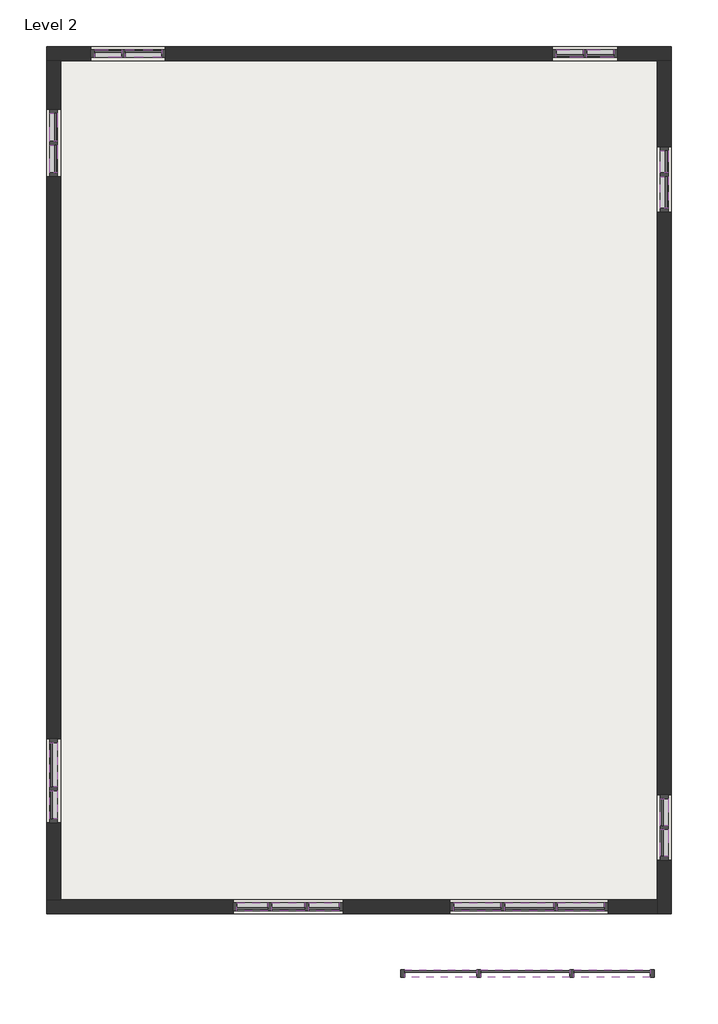
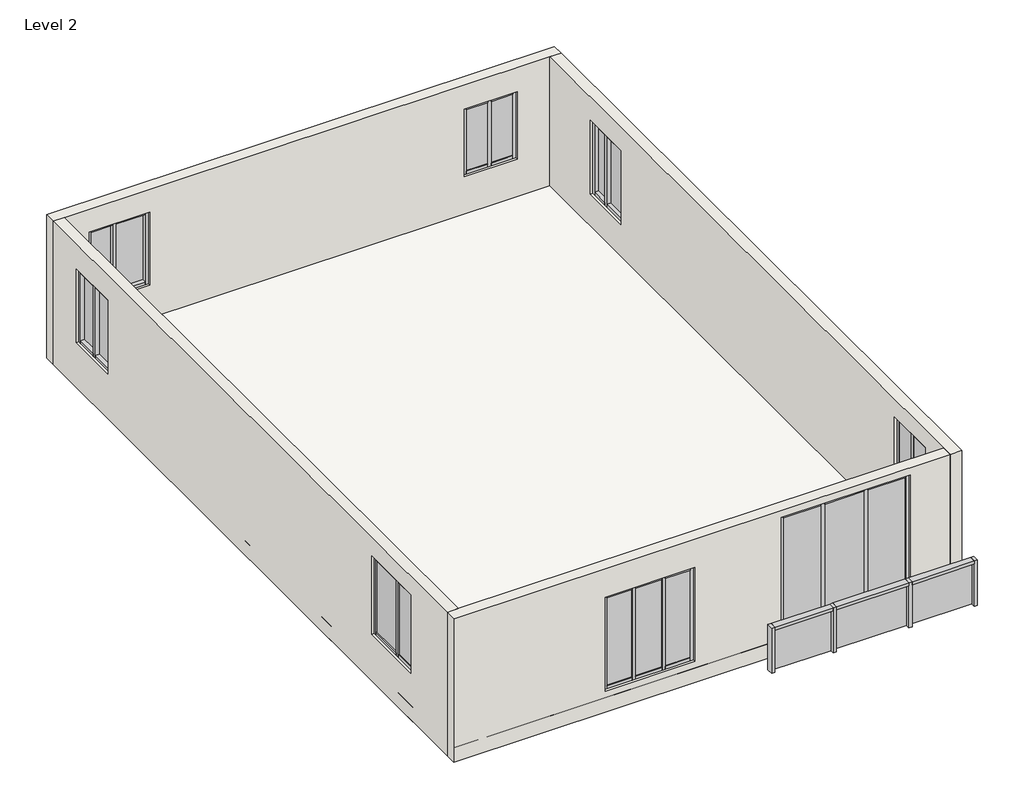
# One storey: 69 members, 21 plates, 4 walls, 1 roof.
"""IFC4 building model written with IfcOpenShell, lengths in millimetres."""

from ifc_helpers import new_model, si_unit, frame, origin, place, context, project, spatial, polyline, outline, extrude, faceted_brep, transform, mapped, element, save
from components import member_e5d39754, member_07406574, member_3ed29256, member_6fb4a552, member_97f07227, member_3e567bd2, member_843225dc, member_0b7646a3, member_1e2e73c0, member_6b6fe981, member_b1e1b578, member_5b6a755a, member_0486e582, member_4eea421a, member_9dbbeca1, member_3cfa9974, member_e7b97c4b, member_5535eeb3, member_7007ad49, member_cfa26838, member_5cb4264a, member_46f5bc36, member_d4df521d, member_0537779b, member_d36207d9, member_2d710983, member_80b18894, member_dd4241ee, member_fb497cbf, member_58cc8d1f, member_066849cb, member_d635bea1, system_panel_glazed_78e3b77e, system_panel_glazed_8adce2ad, system_panel_glazed_79a5eb44, system_panel_glazed_1572ce70, system_panel_glazed_a38fa740, system_panel_glazed_c088aa0a, system_panel_glazed_e446b74d, system_panel_glazed_482dc4ba, system_panel_glazed_bd259d29, system_panel_glazed_c39fb08b, system_panel_glazed_eabd6c1f, system_panel_glazed_831ab98e, system_panel_glazed_4b6d2a40, system_panel_glazed_d871acfc, system_panel_glazed_8bce9487, system_panel_glazed_361cf07d

model = new_model("IFC4")

# Units and contexts
model_context = context("Model", 3, world=origin())
ifc_project = project(units=[si_unit("LENGTHUNIT", "METRE", prefix="MILLI")], contexts=[model_context])

# Site, building, storey
site = spatial("IfcSite", under=ifc_project)
building = spatial("IfcBuilding", under=site)
storey = spatial("IfcBuildingStorey", under=building, Name="Level 2", Elevation=3048.0)

# Members
placement = place(None, origin())
member_shape = member_e5d39754(model_context)
element("IfcMember", 1, ObjectType="Rectangular Mullion : 2.5\" x 5\" rectangular", at=placement, inside=storey, context=model_context, shape_type="MappedRepresentation", body=[
    mapped(member_shape, transform((-15758.7624893, 1071.6959625, 5609.8739989), x_axis=(0.0, 0.0, 1.0), y_axis=(0.0, -1.0, 0.0), z_axis=(1.0, 0.0, 0.0))),
])
element("IfcMember", 2, ObjectType="Rectangular Mullion : 2.5\" x 5\" rectangular", at=placement, inside=storey, context=model_context, shape_type="MappedRepresentation", body=[
    mapped(member_shape, transform((-16349.3124893, 1071.6959625, 4052.5030277), x_axis=(0.0, 0.0, -1.0), y_axis=(0.0, -1.0, 0.0), z_axis=(-1.0, 0.0, 0.0))),
])
member_2_shape = member_07406574(model_context)
element("IfcMember", 3, ObjectType="Rectangular Mullion : 2.5\" x 5\" rectangular", at=placement, inside=storey, context=model_context, shape_type="MappedRepresentation", body=[
    mapped(member_2_shape, transform((-13356.3458226, -12872.9040375, 5485.7911654), x_axis=(0.0, 0.0, 1.0), y_axis=(0.0, 1.0, 0.0), z_axis=(-1.0, 0.0, 0.0))),
])
element("IfcMember", 4, ObjectType="Rectangular Mullion : 2.5\" x 5\" rectangular", at=placement, inside=storey, context=model_context, shape_type="MappedRepresentation", body=[
    mapped(member_2_shape, transform((-14526.8624893, -12872.9040375, 5485.7911654), x_axis=(0.0, 0.0, 1.0), y_axis=(0.0, 1.0, 0.0), z_axis=(-1.0, 0.0, 0.0))),
])
member_3_shape = member_3ed29256(model_context)
element("IfcMember", 5, ObjectType="Rectangular Mullion : 2.5\" x 5\" rectangular", at=placement, inside=storey, context=model_context, shape_type="MappedRepresentation", body=[
    mapped(member_3_shape, transform((-13957.479156, -12872.9040375, 5485.7911654), x_axis=(0.0, 0.0, 1.0), y_axis=(0.0, 1.0, 0.0), z_axis=(-1.0, 0.0, 0.0))),
])
element("IfcMember", 6, ObjectType="Rectangular Mullion : 2.5\" x 5\" rectangular", at=placement, inside=storey, context=model_context, shape_type="MappedRepresentation", body=[
    mapped(member_3_shape, transform((-13419.8458226, -12872.9040375, 3489.9238444), x_axis=(0.0, 0.0, -1.0), y_axis=(0.0, 1.0, 0.0), z_axis=(1.0, 0.0, 0.0))),
])
element("IfcMember", 7, ObjectType="Rectangular Mullion : 2.5\" x 5\" rectangular", at=placement, inside=storey, context=model_context, shape_type="MappedRepresentation", body=[
    mapped(member_2_shape, transform((-14020.979156, -12872.9040375, 3489.9238444), x_axis=(0.0, 0.0, -1.0), y_axis=(0.0, 1.0, 0.0), z_axis=(1.0, 0.0, 0.0))),
])
element("IfcMember", 8, ObjectType="Rectangular Mullion : 2.5\" x 5\" rectangular", at=placement, inside=storey, context=model_context, shape_type="MappedRepresentation", body=[
    mapped(member_2_shape, transform((-12850.4624893, -12872.9040375, 3489.9238444), x_axis=(0.0, 0.0, -1.0), y_axis=(0.0, 1.0, 0.0), z_axis=(1.0, 0.0, 0.0))),
])
member_4_shape = member_6fb4a552(model_context)
element("IfcMember", 9, ObjectType="Rectangular Mullion : 2.5\" x 5\" rectangular", at=placement, inside=storey, context=model_context, shape_type="MappedRepresentation", body=[
    mapped(member_4_shape, transform((-7541.8624893, -11609.2540375, 5711.9340524), x_axis=(0.0, 0.0, 1.0), y_axis=(1.0, 0.0, 0.0), z_axis=(0.0, 1.0, 0.0))),
])
element("IfcMember", 10, ObjectType="Rectangular Mullion : 2.5\" x 5\" rectangular", at=placement, inside=storey, context=model_context, shape_type="MappedRepresentation", body=[
    mapped(member_4_shape, transform((-7541.8624893, -11107.6040375, 5711.9340524), x_axis=(0.0, 0.0, 1.0), y_axis=(1.0, 0.0, 0.0), z_axis=(0.0, 1.0, 0.0))),
])
element("IfcMember", 11, ObjectType="Rectangular Mullion : 2.5\" x 5\" rectangular", at=placement, inside=storey, context=model_context, shape_type="MappedRepresentation", body=[
    mapped(member_4_shape, transform((-8805.5124893, 1071.6959625, 5579.9993984), x_axis=(0.0, 0.0, 1.0), y_axis=(0.0, 1.0, 0.0), z_axis=(-1.0, 0.0, 0.0))),
])
element("IfcMember", 12, ObjectType="Rectangular Mullion : 2.5\" x 5\" rectangular", at=placement, inside=storey, context=model_context, shape_type="MappedRepresentation", body=[
    mapped(member_4_shape, transform((-9307.1624893, 1071.6959625, 5579.9993984), x_axis=(0.0, 0.0, 1.0), y_axis=(0.0, 1.0, 0.0), z_axis=(-1.0, 0.0, 0.0))),
])
element("IfcMember", 13, ObjectType="Rectangular Mullion : 2.5\" x 5\" rectangular", at=placement, inside=storey, context=model_context, shape_type="MappedRepresentation", body=[
    mapped(member_4_shape, transform((-16412.8124893, 1071.6959625, 5609.8739989), x_axis=(0.0, 0.0, 1.0), y_axis=(0.0, -1.0, 0.0), z_axis=(1.0, 0.0, 0.0))),
])
member_5_shape = member_97f07227(model_context)
element("IfcMember", 14, ObjectType="Rectangular Mullion : 2.5\" x 5\" rectangular", at=placement, inside=storey, context=model_context, shape_type="MappedRepresentation", body=[
    mapped(member_5_shape, transform((-7541.8624893, -11577.5040375, 4161.6494696), x_axis=(0.0, 1.0, 0.0), y_axis=(1.0, 0.0, 0.0), z_axis=(0.0, 0.0, -1.0))),
])
element("IfcMember", 15, ObjectType="Rectangular Mullion : 2.5\" x 5\" rectangular", at=placement, inside=storey, context=model_context, shape_type="MappedRepresentation", body=[
    mapped(member_4_shape, transform((-7541.8624893, -11545.7540375, 4161.6494696), x_axis=(0.0, 0.0, -1.0), y_axis=(1.0, 0.0, 0.0), z_axis=(0.0, -1.0, 0.0))),
])
element("IfcMember", 16, ObjectType="Rectangular Mullion : 2.5\" x 5\" rectangular", at=placement, inside=storey, context=model_context, shape_type="MappedRepresentation", body=[
    mapped(member_4_shape, transform((-7541.8624893, -12047.4040375, 4161.6494696), x_axis=(0.0, 0.0, -1.0), y_axis=(1.0, 0.0, 0.0), z_axis=(0.0, -1.0, 0.0))),
])
element("IfcMember", 17, ObjectType="Rectangular Mullion : 2.5\" x 5\" rectangular", at=placement, inside=storey, context=model_context, shape_type="MappedRepresentation", body=[
    mapped(member_4_shape, transform((-8869.0124893, 1071.6959625, 4146.229298), x_axis=(0.0, 0.0, -1.0), y_axis=(0.0, 1.0, 0.0), z_axis=(1.0, 0.0, 0.0))),
])
element("IfcMember", 18, ObjectType="Rectangular Mullion : 2.5\" x 5\" rectangular", at=placement, inside=storey, context=model_context, shape_type="MappedRepresentation", body=[
    mapped(member_4_shape, transform((-8367.3624893, 1071.6959625, 4146.229298), x_axis=(0.0, 0.0, -1.0), y_axis=(0.0, 1.0, 0.0), z_axis=(1.0, 0.0, 0.0))),
])
element("IfcMember", 19, ObjectType="Rectangular Mullion : 2.5\" x 5\" rectangular", at=placement, inside=storey, context=model_context, shape_type="MappedRepresentation", body=[
    mapped(member_4_shape, transform((-16850.9624893, 1071.6959625, 4052.5030277), x_axis=(0.0, 0.0, -1.0), y_axis=(0.0, -1.0, 0.0), z_axis=(-1.0, 0.0, 0.0))),
])
member_6_shape = member_3e567bd2(model_context)
element("IfcMember", 20, ObjectType="Rectangular Mullion : 2.5\" x 5\" rectangular", at=placement, inside=storey, context=model_context, shape_type="MappedRepresentation", body=[
    mapped(member_6_shape, transform((-7541.8624893, -11044.1040375, 4161.6494696), x_axis=(0.0, 1.0, 0.0), y_axis=(1.0, 0.0, 0.0), z_axis=(0.0, 0.0, -1.0))),
])
element("IfcMember", 21, ObjectType="Rectangular Mullion : 2.5\" x 5\" rectangular", at=placement, inside=storey, context=model_context, shape_type="MappedRepresentation", body=[
    mapped(member_6_shape, transform((-7541.8624893, -12110.9040375, 5711.9340524), x_axis=(0.0, -1.0, 0.0), y_axis=(1.0, 0.0, 0.0), z_axis=(0.0, 0.0, 1.0))),
])
member_7_shape = member_843225dc(model_context)
element("IfcMember", 22, ObjectType="Rectangular Mullion : 2.5\" x 5\" rectangular", at=placement, inside=storey, context=model_context, shape_type="MappedRepresentation", body=[
    mapped(member_7_shape, transform((-7541.8624893, -877.7540375, 5599.6032414), x_axis=(0.0, 0.0, 1.0), y_axis=(-1.0, 0.0, 0.0), z_axis=(0.0, -1.0, 0.0))),
])
member_8_shape = member_0b7646a3(model_context)
element("IfcMember", 23, ObjectType="Rectangular Mullion : 2.5\" x 5\" rectangular", at=placement, inside=storey, context=model_context, shape_type="MappedRepresentation", body=[
    mapped(member_8_shape, transform((-7541.8624893, -1455.6040375, 5599.6032414), x_axis=(0.0, 0.0, 1.0), y_axis=(-1.0, 0.0, 0.0), z_axis=(0.0, -1.0, 0.0))),
])
member_9_shape = member_1e2e73c0(model_context)
element("IfcMember", 24, ObjectType="Rectangular Mullion : 2.5\" x 5\" rectangular", at=placement, inside=storey, context=model_context, shape_type="MappedRepresentation", body=[
    mapped(member_9_shape, transform((-7541.8624893, -909.5040375, 4029.8396627), x_axis=(0.0, -1.0, 0.0), y_axis=(-1.0, 0.0, 0.0), z_axis=(0.0, 0.0, -1.0))),
])
element("IfcMember", 25, ObjectType="Rectangular Mullion : 2.5\" x 5\" rectangular", at=placement, inside=storey, context=model_context, shape_type="MappedRepresentation", body=[
    mapped(member_8_shape, transform((-7541.8624893, -941.2540375, 4029.8396627), x_axis=(0.0, 0.0, -1.0), y_axis=(-1.0, 0.0, 0.0), z_axis=(0.0, 1.0, 0.0))),
])
element("IfcMember", 26, ObjectType="Rectangular Mullion : 2.5\" x 5\" rectangular", at=placement, inside=storey, context=model_context, shape_type="MappedRepresentation", body=[
    mapped(member_7_shape, transform((-7541.8624893, -515.8040375, 4029.8396627), x_axis=(0.0, 0.0, -1.0), y_axis=(-1.0, 0.0, 0.0), z_axis=(0.0, 1.0, 0.0))),
])
member_10_shape = member_6b6fe981(model_context)
element("IfcMember", 27, ObjectType="Rectangular Mullion : 2.5\" x 5\" rectangular", at=placement, inside=storey, context=model_context, shape_type="MappedRepresentation", body=[
    mapped(member_10_shape, transform((-7541.8624893, -452.3040375, 5599.6032414), x_axis=(0.0, 1.0, 0.0), y_axis=(-1.0, 0.0, 0.0), z_axis=(0.0, 0.0, 1.0))),
])
element("IfcMember", 28, ObjectType="Rectangular Mullion : 2.5\" x 5\" rectangular", at=placement, inside=storey, context=model_context, shape_type="MappedRepresentation", body=[
    mapped(member_10_shape, transform((-7541.8624893, -1519.1040375, 4029.8396627), x_axis=(0.0, -1.0, 0.0), y_axis=(-1.0, 0.0, 0.0), z_axis=(0.0, 0.0, -1.0))),
])
member_11_shape = member_b1e1b578(model_context)
element("IfcMember", 29, ObjectType="Rectangular Mullion : 2.5\" x 5\" rectangular", at=placement, inside=storey, context=model_context, shape_type="MappedRepresentation", body=[
    mapped(member_11_shape, transform((-8837.2624893, 1071.6959625, 4146.229298), x_axis=(-1.0, 0.0, 0.0), y_axis=(0.0, 1.0, 0.0), z_axis=(0.0, 0.0, -1.0))),
])
member_12_shape = member_5b6a755a(model_context)
element("IfcMember", 30, ObjectType="Rectangular Mullion : 2.5\" x 5\" rectangular", at=placement, inside=storey, context=model_context, shape_type="MappedRepresentation", body=[
    mapped(member_12_shape, transform((-9370.6624893, 1071.6959625, 4146.229298), x_axis=(-1.0, 0.0, 0.0), y_axis=(0.0, 1.0, 0.0), z_axis=(0.0, 0.0, -1.0))),
])
element("IfcMember", 31, ObjectType="Rectangular Mullion : 2.5\" x 5\" rectangular", at=placement, inside=storey, context=model_context, shape_type="MappedRepresentation", body=[
    mapped(member_12_shape, transform((-8303.8624893, 1071.6959625, 5579.9993984), x_axis=(1.0, 0.0, 0.0), y_axis=(0.0, 1.0, 0.0), z_axis=(0.0, 0.0, 1.0))),
])
member_13_shape = member_0486e582(model_context)
element("IfcMember", 32, ObjectType="Rectangular Mullion : 2.5\" x 5\" rectangular", at=placement, inside=storey, context=model_context, shape_type="MappedRepresentation", body=[
    mapped(member_13_shape, transform((-16381.0624893, 1071.6959625, 4052.5030277), x_axis=(1.0, 0.0, 0.0), y_axis=(0.0, -1.0, 0.0), z_axis=(0.0, 0.0, -1.0))),
])
member_14_shape = member_4eea421a(model_context)
element("IfcMember", 33, ObjectType="Rectangular Mullion : 2.5\" x 5\" rectangular", at=placement, inside=storey, context=model_context, shape_type="MappedRepresentation", body=[
    mapped(member_14_shape, transform((-16914.4624893, 1071.6959625, 5609.8739989), x_axis=(-1.0, 0.0, 0.0), y_axis=(0.0, -1.0, 0.0), z_axis=(0.0, 0.0, 1.0))),
])
element("IfcMember", 34, ObjectType="Rectangular Mullion : 2.5\" x 5\" rectangular", at=placement, inside=storey, context=model_context, shape_type="MappedRepresentation", body=[
    mapped(member_14_shape, transform((-15695.2624893, 1071.6959625, 4052.5030277), x_axis=(1.0, 0.0, 0.0), y_axis=(0.0, -1.0, 0.0), z_axis=(0.0, 0.0, -1.0))),
])
member_15_shape = member_9dbbeca1(model_context)
element("IfcMember", 35, ObjectType="Rectangular Mullion : 2.5\" x 5\" rectangular", at=placement, inside=storey, context=model_context, shape_type="MappedRepresentation", body=[
    mapped(member_15_shape, transform((-17524.0624893, -360.2290375, 5564.8264528), x_axis=(0.0, 0.0, 1.0), y_axis=(-1.0, 0.0, 0.0), z_axis=(0.0, -1.0, 0.0))),
])
element("IfcMember", 36, ObjectType="Rectangular Mullion : 2.5\" x 5\" rectangular", at=placement, inside=storey, context=model_context, shape_type="MappedRepresentation", body=[
    mapped(member_15_shape, transform((-17524.0624893, -877.7540375, 5564.8264528), x_axis=(0.0, 0.0, 1.0), y_axis=(-1.0, 0.0, 0.0), z_axis=(0.0, -1.0, 0.0))),
])
member_16_shape = member_3cfa9974(model_context)
element("IfcMember", 37, ObjectType="Rectangular Mullion : 2.5\" x 5\" rectangular", at=placement, inside=storey, context=model_context, shape_type="MappedRepresentation", body=[
    mapped(member_16_shape, transform((-17524.0624893, -391.9790375, 3995.7999113), x_axis=(0.0, -1.0, 0.0), y_axis=(-1.0, 0.0, 0.0), z_axis=(0.0, 0.0, -1.0))),
])
element("IfcMember", 38, ObjectType="Rectangular Mullion : 2.5\" x 5\" rectangular", at=placement, inside=storey, context=model_context, shape_type="MappedRepresentation", body=[
    mapped(member_15_shape, transform((-17524.0624893, -423.7290375, 3995.7999113), x_axis=(0.0, 0.0, -1.0), y_axis=(-1.0, 0.0, 0.0), z_axis=(0.0, 1.0, 0.0))),
])
element("IfcMember", 39, ObjectType="Rectangular Mullion : 2.5\" x 5\" rectangular", at=placement, inside=storey, context=model_context, shape_type="MappedRepresentation", body=[
    mapped(member_15_shape, transform((-17524.0624893, 93.7959625, 3995.7999113), x_axis=(0.0, 0.0, -1.0), y_axis=(-1.0, 0.0, 0.0), z_axis=(0.0, 1.0, 0.0))),
])
member_17_shape = member_e7b97c4b(model_context)
element("IfcMember", 40, ObjectType="Rectangular Mullion : 2.5\" x 5\" rectangular", at=placement, inside=storey, context=model_context, shape_type="MappedRepresentation", body=[
    mapped(member_17_shape, transform((-17524.0624893, -941.2540375, 3995.7999113), x_axis=(0.0, -1.0, 0.0), y_axis=(-1.0, 0.0, 0.0), z_axis=(0.0, 0.0, -1.0))),
])
element("IfcMember", 41, ObjectType="Rectangular Mullion : 2.5\" x 5\" rectangular", at=placement, inside=storey, context=model_context, shape_type="MappedRepresentation", body=[
    mapped(member_17_shape, transform((-17524.0624893, 157.2959625, 5564.8264528), x_axis=(0.0, 1.0, 0.0), y_axis=(-1.0, 0.0, 0.0), z_axis=(0.0, 0.0, 1.0))),
])
member_18_shape = member_5535eeb3(model_context)
element("IfcMember", 42, ObjectType="Rectangular Mullion : 2.5\" x 5\" rectangular", at=placement, inside=storey, context=model_context, shape_type="MappedRepresentation", body=[
    mapped(member_18_shape, transform((-17524.0624893, -10974.2540375, 5698.7553745), x_axis=(0.0, 0.0, 1.0), y_axis=(1.0, 0.0, 0.0), z_axis=(0.0, 1.0, 0.0))),
])
member_19_shape = member_7007ad49(model_context)
element("IfcMember", 43, ObjectType="Rectangular Mullion : 2.5\" x 5\" rectangular", at=placement, inside=storey, context=model_context, shape_type="MappedRepresentation", body=[
    mapped(member_19_shape, transform((-17524.0624893, -10193.2040375, 5698.7553745), x_axis=(0.0, 0.0, 1.0), y_axis=(1.0, 0.0, 0.0), z_axis=(0.0, 1.0, 0.0))),
])
member_20_shape = member_cfa26838(model_context)
element("IfcMember", 44, ObjectType="Rectangular Mullion : 2.5\" x 5\" rectangular", at=placement, inside=storey, context=model_context, shape_type="MappedRepresentation", body=[
    mapped(member_20_shape, transform((-17524.0624893, -10942.5040375, 4032.9560025), x_axis=(0.0, 1.0, 0.0), y_axis=(1.0, 0.0, 0.0), z_axis=(0.0, 0.0, -1.0))),
])
element("IfcMember", 45, ObjectType="Rectangular Mullion : 2.5\" x 5\" rectangular", at=placement, inside=storey, context=model_context, shape_type="MappedRepresentation", body=[
    mapped(member_19_shape, transform((-17524.0624893, -10910.7540375, 4032.9560025), x_axis=(0.0, 0.0, -1.0), y_axis=(1.0, 0.0, 0.0), z_axis=(0.0, -1.0, 0.0))),
])
element("IfcMember", 46, ObjectType="Rectangular Mullion : 2.5\" x 5\" rectangular", at=placement, inside=storey, context=model_context, shape_type="MappedRepresentation", body=[
    mapped(member_18_shape, transform((-17524.0624893, -11437.8040375, 4032.9560025), x_axis=(0.0, 0.0, -1.0), y_axis=(1.0, 0.0, 0.0), z_axis=(0.0, -1.0, 0.0))),
])
member_21_shape = member_5cb4264a(model_context)
element("IfcMember", 47, ObjectType="Rectangular Mullion : 2.5\" x 5\" rectangular", at=placement, inside=storey, context=model_context, shape_type="MappedRepresentation", body=[
    mapped(member_21_shape, transform((-17524.0624893, -11501.3040375, 5698.7553745), x_axis=(0.0, -1.0, 0.0), y_axis=(1.0, 0.0, 0.0), z_axis=(0.0, 0.0, 1.0))),
])
element("IfcMember", 48, ObjectType="Rectangular Mullion : 2.5\" x 5\" rectangular", at=placement, inside=storey, context=model_context, shape_type="MappedRepresentation", body=[
    mapped(member_21_shape, transform((-17524.0624893, -10129.7040375, 4032.9560025), x_axis=(0.0, 1.0, 0.0), y_axis=(1.0, 0.0, 0.0), z_axis=(0.0, 0.0, -1.0))),
])
member_22_shape = member_46f5bc36(model_context)
element("IfcMember", 49, ObjectType="Rectangular Mullion : 2.5\" x 5\" rectangular", at=placement, inside=storey, context=model_context, shape_type="MappedRepresentation", body=[
    mapped(member_22_shape, transform((-9288.1124893, -12872.9040375, 5944.1398762), x_axis=(0.0, 0.0, 1.0), y_axis=(0.0, 1.0, 0.0), z_axis=(-1.0, 0.0, 0.0))),
])
element("IfcMember", 50, ObjectType="Rectangular Mullion : 2.5\" x 5\" rectangular", at=placement, inside=storey, context=model_context, shape_type="MappedRepresentation", body=[
    mapped(member_22_shape, transform((-10983.5624893, -12872.9040375, 5944.1398762), x_axis=(0.0, 0.0, 1.0), y_axis=(0.0, 1.0, 0.0), z_axis=(-1.0, 0.0, 0.0))),
])
member_23_shape = member_d4df521d(model_context)
element("IfcMember", 51, ObjectType="Rectangular Mullion : 2.5\" x 5\" rectangular", at=placement, inside=storey, context=model_context, shape_type="MappedRepresentation", body=[
    mapped(member_23_shape, transform((-10183.4624893, -12872.9040375, 3475.7949453), x_axis=(-1.0, 0.0, 0.0), y_axis=(0.0, 1.0, 0.0), z_axis=(0.0, 0.0, -1.0))),
])
element("IfcMember", 52, ObjectType="Rectangular Mullion : 2.5\" x 5\" rectangular", at=placement, inside=storey, context=model_context, shape_type="MappedRepresentation", body=[
    mapped(member_23_shape, transform((-9319.8624893, -12872.9040375, 3475.7949453), x_axis=(-1.0, 0.0, 0.0), y_axis=(0.0, 1.0, 0.0), z_axis=(0.0, 0.0, -1.0))),
])
element("IfcMember", 53, ObjectType="Rectangular Mullion : 2.5\" x 5\" rectangular", at=placement, inside=storey, context=model_context, shape_type="MappedRepresentation", body=[
    mapped(member_22_shape, transform((-10215.2124893, -12872.9040375, 3475.7949453), x_axis=(0.0, 0.0, -1.0), y_axis=(0.0, 1.0, 0.0), z_axis=(1.0, 0.0, 0.0))),
])
element("IfcMember", 54, ObjectType="Rectangular Mullion : 2.5\" x 5\" rectangular", at=placement, inside=storey, context=model_context, shape_type="MappedRepresentation", body=[
    mapped(member_22_shape, transform((-8519.7624893, -12872.9040375, 3475.7949453), x_axis=(0.0, 0.0, -1.0), y_axis=(0.0, 1.0, 0.0), z_axis=(1.0, 0.0, 0.0))),
])
member_24_shape = member_0537779b(model_context)
element("IfcMember", 55, ObjectType="Rectangular Mullion : 2.5\" x 5\" rectangular", at=placement, inside=storey, context=model_context, shape_type="MappedRepresentation", body=[
    mapped(member_24_shape, transform((-11047.0624893, -12872.9040375, 3475.7949453), x_axis=(-1.0, 0.0, 0.0), y_axis=(0.0, 1.0, 0.0), z_axis=(0.0, 0.0, -1.0))),
])
member_25_shape = member_d36207d9(model_context)
element("IfcMember", 56, ObjectType="Rectangular Mullion : 2.5\" x 5\" rectangular", at=placement, inside=storey, context=model_context, shape_type="MappedRepresentation", body=[
    mapped(member_25_shape, transform((-10151.7124893, -12872.9040375, 5944.1398762), x_axis=(0.0, 0.0, 1.0), y_axis=(0.0, 1.0, 0.0), z_axis=(-1.0, 0.0, 0.0))),
])
element("IfcMember", 57, ObjectType="Rectangular Mullion : 2.5\" x 5\" rectangular", at=placement, inside=storey, context=model_context, shape_type="MappedRepresentation", body=[
    mapped(member_25_shape, transform((-9351.6124893, -12872.9040375, 3475.7949453), x_axis=(0.0, 0.0, -1.0), y_axis=(0.0, 1.0, 0.0), z_axis=(1.0, 0.0, 0.0))),
])
element("IfcMember", 58, ObjectType="Rectangular Mullion : 2.5\" x 5\" rectangular", at=placement, inside=storey, context=model_context, shape_type="MappedRepresentation", body=[
    mapped(member_24_shape, transform((-8456.2624893, -12872.9040375, 5944.1398762), x_axis=(1.0, 0.0, 0.0), y_axis=(0.0, 1.0, 0.0), z_axis=(0.0, 0.0, 1.0))),
])
member_26_shape = member_2d710983(model_context)
element("IfcMember", 59, ObjectType="Rectangular Mullion : 2.5\" x 5\" rectangular", at=placement, inside=storey, context=model_context, shape_type="MappedRepresentation", body=[
    mapped(member_26_shape, transform((-13989.229156, -12872.9040375, 3489.9238444), x_axis=(-1.0, 0.0, 0.0), y_axis=(0.0, 1.0, 0.0), z_axis=(0.0, 0.0, -1.0))),
])
element("IfcMember", 60, ObjectType="Rectangular Mullion : 2.5\" x 5\" rectangular", at=placement, inside=storey, context=model_context, shape_type="MappedRepresentation", body=[
    mapped(member_26_shape, transform((-13388.0958226, -12872.9040375, 3489.9238444), x_axis=(-1.0, 0.0, 0.0), y_axis=(0.0, 1.0, 0.0), z_axis=(0.0, 0.0, -1.0))),
])
member_27_shape = member_80b18894(model_context)
element("IfcMember", 61, ObjectType="Rectangular Mullion : 2.5\" x 5\" rectangular", at=placement, inside=storey, context=model_context, shape_type="MappedRepresentation", body=[
    mapped(member_27_shape, transform((-12786.9624893, -12872.9040375, 5485.7911654), x_axis=(1.0, 0.0, 0.0), y_axis=(0.0, 1.0, 0.0), z_axis=(0.0, 0.0, 1.0))),
])
element("IfcMember", 62, ObjectType="Rectangular Mullion : 2.5\" x 5\" rectangular", at=placement, inside=storey, context=model_context, shape_type="MappedRepresentation", body=[
    mapped(member_27_shape, transform((-14590.3624893, -12872.9040375, 3489.9238444), x_axis=(-1.0, 0.0, 0.0), y_axis=(0.0, 1.0, 0.0), z_axis=(0.0, 0.0, -1.0))),
])
member_28_shape = member_dd4241ee(model_context)
element("IfcMember", 63, ObjectType="Rectangular Mullion : 2.5\" x 5\" rectangular", at=placement, inside=storey, context=model_context, shape_type="MappedRepresentation", body=[
    mapped(member_28_shape, transform((-11847.1624893, -13965.1040375, 4500.0986575), x_axis=(-1.0, 0.0, 0.0), y_axis=(0.0, -1.0, 0.0), z_axis=(0.0, 0.0, 1.0))),
])
member_29_shape = member_fb497cbf(model_context)
element("IfcMember", 64, ObjectType="Rectangular Mullion : 2.5\" x 5\" rectangular", at=placement, inside=storey, context=model_context, shape_type="MappedRepresentation", body=[
    mapped(member_29_shape, transform((-10608.9124893, -13965.1040375, 4500.0986575), x_axis=(0.0, 0.0, 1.0), y_axis=(0.0, -1.0, 0.0), z_axis=(1.0, 0.0, 0.0))),
])
member_30_shape = member_58cc8d1f(model_context)
element("IfcMember", 65, ObjectType="Rectangular Mullion : 2.5\" x 5\" rectangular", at=placement, inside=storey, context=model_context, shape_type="MappedRepresentation", body=[
    mapped(member_30_shape, transform((-10577.1624893, -13965.1040375, 3539.2949453), x_axis=(1.0, 0.0, 0.0), y_axis=(0.0, -1.0, 0.0), z_axis=(0.0, 0.0, -1.0))),
])
element("IfcMember", 66, ObjectType="Rectangular Mullion : 2.5\" x 5\" rectangular", at=placement, inside=storey, context=model_context, shape_type="MappedRepresentation", body=[
    mapped(member_30_shape, transform((-9055.2871232, -13965.1040375, 3539.2949453), x_axis=(1.0, 0.0, 0.0), y_axis=(0.0, -1.0, 0.0), z_axis=(0.0, 0.0, -1.0))),
])
member_31_shape = member_066849cb(model_context)
element("IfcMember", 67, ObjectType="Rectangular Mullion : 2.5\" x 5\" rectangular", at=placement, inside=storey, context=model_context, shape_type="MappedRepresentation", body=[
    mapped(member_31_shape, transform((-9087.0371232, -13965.1040375, 4500.0986575), x_axis=(0.0, 0.0, 1.0), y_axis=(0.0, -1.0, 0.0), z_axis=(1.0, 0.0, 0.0))),
])
member_32_shape = member_d635bea1(model_context)
element("IfcMember", 68, ObjectType="Rectangular Mullion : 2.5\" x 5\" rectangular", at=placement, inside=storey, context=model_context, shape_type="MappedRepresentation", body=[
    mapped(member_32_shape, transform((-7772.5871232, -13965.1040375, 4500.0986575), x_axis=(0.0, 0.0, 1.0), y_axis=(0.0, -1.0, 0.0), z_axis=(1.0, 0.0, 0.0))),
])
element("IfcMember", 69, ObjectType="Rectangular Mullion : 2.5\" x 5\" rectangular", at=placement, inside=storey, context=model_context, shape_type="MappedRepresentation", body=[
    mapped(member_28_shape, transform((-7709.0871232, -13965.1040375, 3539.2949453), x_axis=(1.0, 0.0, 0.0), y_axis=(0.0, -1.0, 0.0), z_axis=(0.0, 0.0, -1.0))),
])

# Plates
system_panel_glazed_shape = system_panel_glazed_78e3b77e(model_context)
element("IfcPlate", 70, ObjectType="System Panel : Glazed", at=placement, inside=storey, context=model_context, shape_type="MappedRepresentation", body=[
    mapped(system_panel_glazed_shape, transform((-7541.8624893, -11828.3290375, 4225.1494696), x_axis=(0.0, 1.0, 0.0), y_axis=(-1.0, 0.0, 0.0), z_axis=(0.0, 0.0, 1.0))),
])
element("IfcPlate", 71, ObjectType="System Panel : Glazed", at=placement, inside=storey, context=model_context, shape_type="MappedRepresentation", body=[
    mapped(system_panel_glazed_shape, transform((-7541.8624893, -11326.6790375, 4225.1494696), x_axis=(0.0, 1.0, 0.0), y_axis=(-1.0, 0.0, 0.0), z_axis=(0.0, 0.0, 1.0))),
])
system_panel_glazed_2_shape = system_panel_glazed_8adce2ad(model_context)
element("IfcPlate", 72, ObjectType="System Panel : Glazed", at=placement, inside=storey, context=model_context, shape_type="MappedRepresentation", body=[
    mapped(system_panel_glazed_2_shape, transform((-7541.8624893, -696.7790375, 4093.3396627), x_axis=(0.0, -1.0, 0.0), y_axis=(1.0, 0.0, 0.0), z_axis=(0.0, 0.0, 1.0))),
])
system_panel_glazed_3_shape = system_panel_glazed_79a5eb44(model_context)
element("IfcPlate", 73, ObjectType="System Panel : Glazed", at=placement, inside=storey, context=model_context, shape_type="MappedRepresentation", body=[
    mapped(system_panel_glazed_3_shape, transform((-7541.8624893, -1198.4290375, 4093.3396627), x_axis=(0.0, -1.0, 0.0), y_axis=(1.0, 0.0, 0.0), z_axis=(0.0, 0.0, 1.0))),
])
system_panel_glazed_4_shape = system_panel_glazed_1572ce70(model_context)
element("IfcPlate", 74, ObjectType="System Panel : Glazed", at=placement, inside=storey, context=model_context, shape_type="MappedRepresentation", body=[
    mapped(system_panel_glazed_4_shape, transform((-8586.4374893, 1071.6959625, 4209.729298), x_axis=(-1.0, 0.0, 0.0), y_axis=(0.0, -1.0, 0.0), z_axis=(0.0, 0.0, 1.0))),
])
element("IfcPlate", 75, ObjectType="System Panel : Glazed", at=placement, inside=storey, context=model_context, shape_type="MappedRepresentation", body=[
    mapped(system_panel_glazed_4_shape, transform((-9088.0874893, 1071.6959625, 4209.729298), x_axis=(-1.0, 0.0, 0.0), y_axis=(0.0, -1.0, 0.0), z_axis=(0.0, 0.0, 1.0))),
])
system_panel_glazed_5_shape = system_panel_glazed_a38fa740(model_context)
element("IfcPlate", 76, ObjectType="System Panel : Glazed", at=placement, inside=storey, context=model_context, shape_type="MappedRepresentation", body=[
    mapped(system_panel_glazed_5_shape, transform((-16631.8874893, 1071.6959625, 4116.0030277), x_axis=(1.0, 0.0, 0.0), y_axis=(0.0, 1.0, 0.0), z_axis=(0.0, 0.0, 1.0))),
])
system_panel_glazed_6_shape = system_panel_glazed_c088aa0a(model_context)
element("IfcPlate", 77, ObjectType="System Panel : Glazed", at=placement, inside=storey, context=model_context, shape_type="MappedRepresentation", body=[
    mapped(system_panel_glazed_6_shape, transform((-16054.0374893, 1071.6959625, 4116.0030277), x_axis=(1.0, 0.0, 0.0), y_axis=(0.0, 1.0, 0.0), z_axis=(0.0, 0.0, 1.0))),
])
system_panel_glazed_7_shape = system_panel_glazed_e446b74d(model_context)
element("IfcPlate", 78, ObjectType="System Panel : Glazed", at=placement, inside=storey, context=model_context, shape_type="MappedRepresentation", body=[
    mapped(system_panel_glazed_7_shape, transform((-17524.0624893, -133.2165375, 4059.2999113), x_axis=(0.0, -1.0, 0.0), y_axis=(1.0, 0.0, 0.0), z_axis=(0.0, 0.0, 1.0))),
])
element("IfcPlate", 79, ObjectType="System Panel : Glazed", at=placement, inside=storey, context=model_context, shape_type="MappedRepresentation", body=[
    mapped(system_panel_glazed_7_shape, transform((-17524.0624893, -650.7415375, 4059.2999113), x_axis=(0.0, -1.0, 0.0), y_axis=(1.0, 0.0, 0.0), z_axis=(0.0, 0.0, 1.0))),
])
system_panel_glazed_8_shape = system_panel_glazed_482dc4ba(model_context)
element("IfcPlate", 80, ObjectType="System Panel : Glazed", at=placement, inside=storey, context=model_context, shape_type="MappedRepresentation", body=[
    mapped(system_panel_glazed_8_shape, transform((-17524.0624893, -11206.0290375, 4096.4560025), x_axis=(0.0, 1.0, 0.0), y_axis=(-1.0, 0.0, 0.0), z_axis=(0.0, 0.0, 1.0))),
])
system_panel_glazed_9_shape = system_panel_glazed_bd259d29(model_context)
element("IfcPlate", 81, ObjectType="System Panel : Glazed", at=placement, inside=storey, context=model_context, shape_type="MappedRepresentation", body=[
    mapped(system_panel_glazed_9_shape, transform((-17524.0624893, -10551.9790375, 4096.4560025), x_axis=(0.0, 1.0, 0.0), y_axis=(-1.0, 0.0, 0.0), z_axis=(0.0, 0.0, 1.0))),
])
system_panel_glazed_10_shape = system_panel_glazed_c39fb08b(model_context)
element("IfcPlate", 82, ObjectType="System Panel : Glazed", at=placement, inside=storey, context=model_context, shape_type="MappedRepresentation", body=[
    mapped(system_panel_glazed_10_shape, transform((-8903.9374893, -12872.9040375, 3539.2949453), x_axis=(-1.0, 0.0, 0.0), y_axis=(0.0, -1.0, 0.0), z_axis=(0.0, 0.0, 1.0))),
])
element("IfcPlate", 83, ObjectType="System Panel : Glazed", at=placement, inside=storey, context=model_context, shape_type="MappedRepresentation", body=[
    mapped(system_panel_glazed_10_shape, transform((-10599.3874893, -12872.9040375, 3539.2949453), x_axis=(-1.0, 0.0, 0.0), y_axis=(0.0, -1.0, 0.0), z_axis=(0.0, 0.0, 1.0))),
])
system_panel_glazed_11_shape = system_panel_glazed_eabd6c1f(model_context)
element("IfcPlate", 84, ObjectType="System Panel : Glazed", at=placement, inside=storey, context=model_context, shape_type="MappedRepresentation", body=[
    mapped(system_panel_glazed_11_shape, transform((-9751.6624893, -12872.9040375, 3539.2949453), x_axis=(-1.0, 0.0, 0.0), y_axis=(0.0, -1.0, 0.0), z_axis=(0.0, 0.0, 1.0))),
])
system_panel_glazed_12_shape = system_panel_glazed_831ab98e(model_context)
element("IfcPlate", 85, ObjectType="System Panel : Glazed", at=placement, inside=storey, context=model_context, shape_type="MappedRepresentation", body=[
    mapped(system_panel_glazed_12_shape, transform((-13103.404156, -12872.9040375, 3553.4238444), x_axis=(-1.0, 0.0, 0.0), y_axis=(0.0, -1.0, 0.0), z_axis=(0.0, 0.0, 1.0))),
])
element("IfcPlate", 86, ObjectType="System Panel : Glazed", at=placement, inside=storey, context=model_context, shape_type="MappedRepresentation", body=[
    mapped(system_panel_glazed_12_shape, transform((-14273.9208226, -12872.9040375, 3553.4238444), x_axis=(-1.0, 0.0, 0.0), y_axis=(0.0, -1.0, 0.0), z_axis=(0.0, 0.0, 1.0))),
])
system_panel_glazed_13_shape = system_panel_glazed_4b6d2a40(model_context)
element("IfcPlate", 87, ObjectType="System Panel : Glazed", at=placement, inside=storey, context=model_context, shape_type="MappedRepresentation", body=[
    mapped(system_panel_glazed_13_shape, transform((-13688.6624893, -12872.9040375, 3553.4238444), x_axis=(-1.0, 0.0, 0.0), y_axis=(0.0, -1.0, 0.0), z_axis=(0.0, 0.0, 1.0))),
])
system_panel_glazed_14_shape = system_panel_glazed_d871acfc(model_context)
element("IfcPlate", 88, ObjectType="System Panel : Glazed", at=placement, inside=storey, context=model_context, shape_type="MappedRepresentation", body=[
    mapped(system_panel_glazed_14_shape, transform((-11196.2874893, -13965.1040375, 3539.2949453), x_axis=(1.0, 0.0, 0.0), y_axis=(0.0, 1.0, 0.0), z_axis=(0.0, 0.0, 1.0))),
])
system_panel_glazed_15_shape = system_panel_glazed_8bce9487(model_context)
element("IfcPlate", 89, ObjectType="System Panel : Glazed", at=placement, inside=storey, context=model_context, shape_type="MappedRepresentation", body=[
    mapped(system_panel_glazed_15_shape, transform((-9816.2248062, -13965.1040375, 3539.2949453), x_axis=(1.0, 0.0, 0.0), y_axis=(0.0, 1.0, 0.0), z_axis=(0.0, 0.0, 1.0))),
])
system_panel_glazed_16_shape = system_panel_glazed_361cf07d(model_context)
element("IfcPlate", 90, ObjectType="System Panel : Glazed", at=placement, inside=storey, context=model_context, shape_type="MappedRepresentation", body=[
    mapped(system_panel_glazed_16_shape, transform((-8398.0621232, -13965.1040375, 3539.2949453), x_axis=(1.0, 0.0, 0.0), y_axis=(0.0, 1.0, 0.0), z_axis=(0.0, 0.0, 1.0))),
])

# Roof
element("IfcRoof", 91, ObjectType="Generic - 12\"", at=placement, inside=storey, context=model_context, shape_type="SweptSolid", body=[
    extrude(outline(polyline([(-17638.3624893, 1185.9959625), (-7427.5624893, 1185.9959625), (-7427.5624893, -12987.2040375), (-17638.3624893, -12987.2040375), (-17638.3624893, 1185.9959625)])), frame((0.0, 0.0, 3048.0), z_axis=(0.0, 0.0, 1.0), x_axis=(1.0, 0.0, 0.0)), (0.0, 0.0, 1.0), 304.8),
])

# Walls
element("IfcWall", 92, ObjectType="9\"", at=placement, inside=storey, context=model_context, shape_type="Brep", body=[
    faceted_brep([(-17638.3624893, 957.3959625, 3048.0), (-17409.7624893, 957.3959625, 3048.0), (-7656.1624893, 957.3959625, 3048.0), (-7427.5624893, 957.3959625, 3048.0), (-7427.5624893, 957.3959625, 6096.0), (-7656.1624893, 957.3959625, 6096.0), (-17409.7624893, 957.3959625, 6096.0), (-17638.3624893, 957.3959625, 6096.0), (-8303.8624893, 957.3959625, 5579.9993984), (-8303.8624893, 957.3959625, 4146.229298), (-9370.6624893, 957.3959625, 4146.229298), (-9370.6624893, 957.3959625, 5579.9993984), (-16914.4624893, 957.3959625, 4052.5030277), (-16914.4624893, 957.3959625, 5609.8739989), (-15695.2624893, 957.3959625, 5609.8739989), (-15695.2624893, 957.3959625, 4052.5030277), (-7427.5624893, 1185.9959625, 3048.0), (-17638.3624893, 1185.9959625, 3048.0), (-17638.3624893, 1185.9959625, 6096.0), (-7427.5624893, 1185.9959625, 6096.0), (-8303.8624893, 1185.9959625, 4146.229298), (-8303.8624893, 1185.9959625, 5579.9993984), (-9370.6624893, 1185.9959625, 5579.9993984), (-9370.6624893, 1185.9959625, 4146.229298), (-16914.4624893, 1185.9959625, 5609.8739989), (-16914.4624893, 1185.9959625, 4052.5030277), (-15695.2624893, 1185.9959625, 4052.5030277), (-15695.2624893, 1185.9959625, 5609.8739989)], [[[0, 1, 2, 3, 4, 5, 6, 7], [8, 9, 10, 11], [12, 13, 14, 15]], [[16, 17, 18, 19], [20, 21, 22, 23], [24, 25, 26, 27]], [[3, 2, 1, 0, 17, 16]], [[7, 6, 5, 4, 19, 18]], [[4, 3, 16, 19]], [[0, 7, 18, 17]], [[8, 21, 20, 9]], [[21, 8, 11, 22]], [[22, 11, 10, 23]], [[9, 20, 23, 10]], [[12, 25, 24, 13]], [[13, 24, 27, 14]], [[14, 27, 26, 15]], [[25, 12, 15, 26]]]),
])
element("IfcWall", 93, ObjectType="9\"", at=placement, inside=storey, context=model_context, shape_type="Brep", body=[
    faceted_brep([(-7656.1624893, 957.3959625, 3048.0), (-7656.1624893, -12758.6040375, 3048.0), (-7656.1624893, -12987.2040375, 3048.0), (-7656.1624893, -12987.2040375, 6096.0), (-7656.1624893, -12758.6040375, 6096.0), (-7656.1624893, 957.3959625, 6096.0), (-7656.1624893, -452.3040375, 4029.8396627), (-7656.1624893, -452.3040375, 5599.6032414), (-7656.1624893, -1519.1040375, 5599.6032414), (-7656.1624893, -1519.1040375, 4029.8396627), (-7656.1624893, -12110.9040375, 5711.9340524), (-7656.1624893, -12110.9040375, 4161.6494696), (-7656.1624893, -11044.1040375, 4161.6494696), (-7656.1624893, -11044.1040375, 5711.9340524), (-7427.5624893, -12987.2040375, 3048.0), (-7427.5624893, 957.3959625, 3048.0), (-7427.5624893, 957.3959625, 6096.0), (-7427.5624893, -12987.2040375, 6096.0), (-7427.5624893, -452.3040375, 5599.6032414), (-7427.5624893, -452.3040375, 4029.8396627), (-7427.5624893, -1519.1040375, 4029.8396627), (-7427.5624893, -1519.1040375, 5599.6032414), (-7427.5624893, -12110.9040375, 4161.6494696), (-7427.5624893, -12110.9040375, 5711.9340524), (-7427.5624893, -11044.1040375, 5711.9340524), (-7427.5624893, -11044.1040375, 4161.6494696)], [[[0, 1, 2, 3, 4, 5], [6, 7, 8, 9], [10, 11, 12, 13]], [[14, 15, 16, 17], [18, 19, 20, 21], [22, 23, 24, 25]], [[2, 1, 0, 15, 14]], [[5, 4, 3, 17, 16]], [[0, 5, 16, 15]], [[3, 2, 14, 17]], [[18, 7, 6, 19]], [[7, 18, 21, 8]], [[8, 21, 20, 9]], [[19, 6, 9, 20]], [[22, 11, 10, 23]], [[23, 10, 13, 24]], [[24, 13, 12, 25]], [[11, 22, 25, 12]]]),
])
element("IfcWall", 94, ObjectType="9\"", at=placement, inside=storey, context=model_context, shape_type="Brep", body=[
    faceted_brep([(-7656.1624893, -12758.6040375, 3048.0), (-17409.7624893, -12758.6040375, 3048.0), (-17638.3624893, -12758.6040375, 3048.0), (-17638.3624893, -12758.6040375, 6096.0), (-17409.7624893, -12758.6040375, 6096.0), (-7656.1624893, -12758.6040375, 6096.0), (-8456.2624893, -12758.6040375, 3475.7949453), (-8456.2624893, -12758.6040375, 5944.1398762), (-11047.0624893, -12758.6040375, 5944.1398762), (-11047.0624893, -12758.6040375, 3475.7949453), (-12786.9624893, -12758.6040375, 3489.9238444), (-12786.9624893, -12758.6040375, 5485.7911654), (-14590.3624893, -12758.6040375, 5485.7911654), (-14590.3624893, -12758.6040375, 3489.9238444), (-17638.3624893, -12987.2040375, 3048.0), (-7656.1624893, -12987.2040375, 3048.0), (-7656.1624893, -12987.2040375, 6096.0), (-17638.3624893, -12987.2040375, 6096.0), (-8456.2624893, -12987.2040375, 5944.1398762), (-8456.2624893, -12987.2040375, 3475.7949453), (-11047.0624893, -12987.2040375, 3475.7949453), (-11047.0624893, -12987.2040375, 5944.1398762), (-12786.9624893, -12987.2040375, 5485.7911654), (-12786.9624893, -12987.2040375, 3489.9238444), (-14590.3624893, -12987.2040375, 3489.9238444), (-14590.3624893, -12987.2040375, 5485.7911654)], [[[0, 1, 2, 3, 4, 5], [6, 7, 8, 9], [10, 11, 12, 13]], [[14, 15, 16, 17], [18, 19, 20, 21], [22, 23, 24, 25]], [[2, 1, 0, 15, 14]], [[5, 4, 3, 17, 16]], [[0, 5, 16, 15]], [[3, 2, 14, 17]], [[18, 7, 6, 19]], [[7, 18, 21, 8]], [[8, 21, 20, 9]], [[19, 6, 9, 20]], [[10, 23, 22, 11]], [[11, 22, 25, 12]], [[12, 25, 24, 13]], [[23, 10, 13, 24]]]),
])
element("IfcWall", 95, ObjectType="9\"", at=placement, inside=storey, context=model_context, shape_type="SweptSolid", body=[
    extrude(outline(polyline([(957.3959625, 3048.0), (-12758.6040375, 3048.0), (-12758.6040375, 6096.0), (957.3959625, 6096.0), (957.3959625, 3048.0)]), holes=[polyline([(157.2959625, 3995.7999113), (157.2959625, 5564.8264528), (-941.2540375, 5564.8264528), (-941.2540375, 3995.7999113), (157.2959625, 3995.7999113)]), polyline([(-11501.3040375, 5698.7553745), (-11501.3040375, 4032.9560025), (-10129.7040375, 4032.9560025), (-10129.7040375, 5698.7553745), (-11501.3040375, 5698.7553745)])]), frame((-17638.3624893, 0.0, 0.0), z_axis=(1.0, 0.0, 0.0), x_axis=(0.0, 1.0, 0.0)), (0.0, 0.0, 1.0), 228.6),
])

save(model, "model.ifc")

# Revit data of these elements
# Type "Rectangular Mullion : 2.5\" x 5\" rectangular"
#   built-in parameter 1007304 = 0.416667 (stored number, unit not read)
#   built-in parameter 1007301 = 0.104167 (stored number, unit not read)
#   built-in parameter 1007300 = 0.104167 (stored number, unit not read)
# Type "System Panel : Glazed"
#   Construction Type Id = "GSP4R"
#   Analytic Construction = "1/8 in Pilkington single glazing"
#   Visual Light Transmittance = 0.9
#   Solar Heat Gain Coefficient = 0.86
#   Heat Transfer Coefficient (U) = 1.18115 BTU/(h·ft²·°F)
#   Define Thermal Properties by = 1
# Type "Generic - 12\""
#   Assembly Code = "B1020"
#   Layers, outside or top first: 1' - 0" no material (function 1)
# Type "9\""
#   Assembly Code = "B2010"
#   Layers, outside or top first: 0' - 9" no material (function 1)
# Elements 1, 2, 3, 4, 5, 6, 7, 8, 9, 10, 11, 12, 13, 14, 15, 16, 17, 18, 19, 20, 21, 22, 23, 24, 25, 26, 27, 28, 29, 30, 31, 32, 33, 34, 35, 36, 37, 38, 39, 40, 41, 42, 43, 44, 45, 46, 47, 48, 49, 50, 51, 52, 53, 54, 55, 56, 57, 58, 59, 60, 61, 62, 63, 64, 65, 66, 67, 68, 69 (IfcMember, "Rectangular Mullion : 2.5\" x 5\" rectangular")
#   Phase Created = New Construction
#   Materials on its faces: "Aluminum"
# Elements 70, 71, 72, 73, 74, 75, 76, 77, 78, 79, 80, 81, 82, 83, 84, 85, 86, 87, 88, 89, 90 (IfcPlate, "System Panel : Glazed")
#   Phase Created = New Construction
#   Materials on its faces: "Glass"
# Element 91 (IfcRoof, "Generic - 12\"")
#   built-in parameter 1001705 = 11 (stored number, unit not read)
#   built-in parameter 1001710 = 33615
#   Phase Created = New Construction
#   Materials on its faces: "Default Roof"
# Elements 92, 93, 94, 95 (IfcWall, "9\"")
#   Top Offset = 0' - 0"
#   Base Offset = 0' - 0"
#   Unconnected Height = 10' - 0"
#   wall height = 10' - 0"
#   Phase Created = New Construction
#   Base Constraint = Level 2
#   Materials on its faces: "Default Wall"
# Materials
#   "Aluminum": class "Metal", colour RGB 247 247 247, transparency 0, Description = "Aluminum 6061", Cost = 0
#   "Glass": class "Glass", colour RGB 0 128 192, transparency 0.75, Description = "Soda Lime Glass", Cost = 0
#   "Default Roof": colour RGB 88 101 114, transparency 0, Cost = 0
#   "Default Wall": colour RGB 128 128 128, transparency 0, Cost = 0
